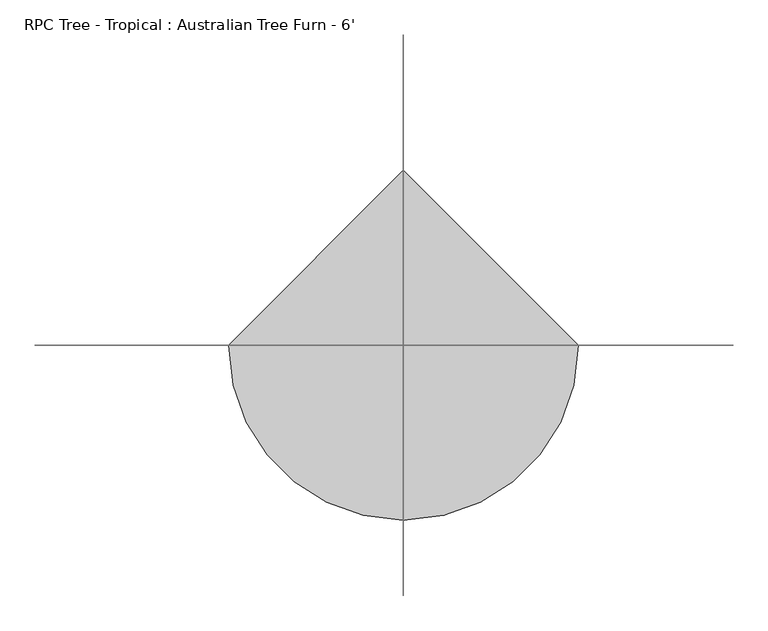
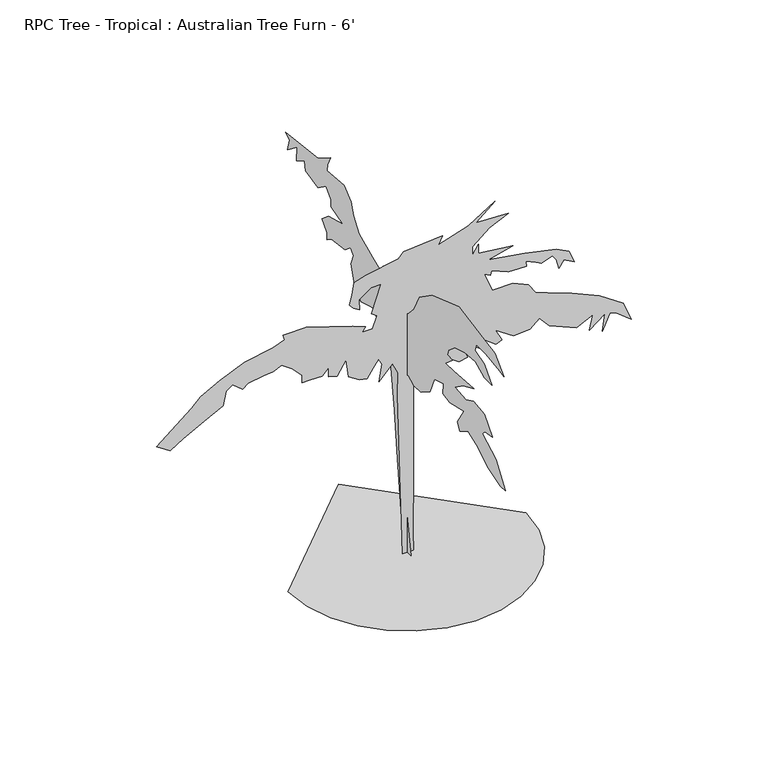
"""IFC4 building model written with IfcOpenShell, lengths in millimetres: geographic element geometry, RPC Tree - Tropical : Australian Tree Furn - 6'."""

from ifc_helpers import new_model, si_unit, origin, place, context, project, spatial, triangles, source, transform, mapped, element, save


def rpc_tree_tropical_australian_tree_furn_6_77f1a640(model_context):
    return source(origin(), model_context, "Body", "Tessellation", [
        triangles([(-639.0365753, 0.0, 0.0007159), (-622.1405136, -146.4247652, 0.0007159), (-574.0277527, -280.8912123, 0.0007159), (-498.5465315, -399.5499215, 0.0007159), (-399.5499215, -498.5465315, 0.0007159), (-280.8912123, -574.0277527, 0.0007159), (-146.4247652, -622.1405136, 0.0007159), (2.79e-05, -639.0365753, 0.0007159), (146.4247652, -622.1429844, 0.0007159), (280.8912123, -574.0277527, 0.0007159), (399.5499215, -498.5465315, 0.0007159), (498.5465315, -399.5499215, 0.0007159), (574.0277527, -280.8912123, 0.0007159), (622.1405136, -146.4247652, 0.0007159), (639.0365753, 5.59e-05, 0.0007159), (-8.38e-05, 639.0365753, 0.0007159), (470.2991641, -3.5e-05, 1828.8014534), (368.5593713, -2.98e-05, 1741.5955845), (542.9711454, -2.94e-05, 1734.3285862), (441.231389, -2.66e-05, 1687.0922253), (350.3907492, -2.2e-05, 1610.7880165), (350.3907492, -1.92e-05, 1563.5516556), (383.0932589, -2.22e-05, 1614.4202076), (383.0932589, -1.92e-05, 1563.5516556), (568.4067295, -1.79e-05, 1541.750806), (437.5966181, -1.59e-05, 1509.0482964), (633.8092781, -1.4e-05, 1476.3456413), (800.9540903, -1.18e-05, 1440.0109406), (869.9913008, -9.7e-06, 1403.673769), (899.0591486, -5.5e-06, 1334.6364132), (840.9235256, -7.5e-06, 1367.3389229), (815.4879416, -5.1e-06, 1327.3695602), (800.9540903, -8.4e-06, 1381.8729195), (779.1532408, -1.01e-05, 1410.9406219), (721.015147, -8.8e-06, 1389.1397724), (691.9473719, -9.7e-06, 1403.673769), (637.4440126, -1.12e-05, 1429.1092804), (641.0762037, -9.4e-06, 1400.0414326), (597.4745047, -9.4e-06, 1400.0414326), (542.9711454, -9.7e-06, 1403.673769), (452.1330491, -1.18e-05, 1440.0109406), (448.4983146, -1.03e-05, 1414.5754292), (415.7958049, -1.14e-05, 1432.7440876), (459.4000111, -5.1e-06, 1327.3695602), (568.4067295, -5.1e-06, 1327.3695602), (651.9778639, -2.9e-06, 1291.0347141), (688.3126373, 3e-07, 1236.5313549), (753.7176567, 1.8e-06, 1211.0958435), (884.5252247, 4.9e-06, 1160.2246754), (1033.5014511, 8.7e-06, 1094.8221268), (1160.6767553, 1.39e-05, 1007.6162579), (1204.2784544, 2.02e-05, 902.2417305), (1120.70732, 1.63e-05, 967.6468225), (1088.0048103, 1.59e-05, 974.9137482), (1048.0353024, 2.11e-05, 887.7078793), (1062.5692263, 1.55e-05, 982.1806738), (978.9980919, 1.94e-05, 916.7781979), (997.1666777, 1.44e-05, 1000.3493322), (909.9608088, 1.7e-05, 956.7450897), (764.6193169, 1.33e-05, 1018.5179907), (710.1159576, 9.6e-06, 1080.2882755), (659.2448622, 1.22e-05, 1036.684033), (572.0389206, 1.26e-05, 1029.4171074), (473.9338986, 8.7e-06, 1094.8221268), (510.2686357, 1.26e-05, 1029.4171074), (477.5660897, 1.35e-05, 1014.8831835), (324.9577085, 6.6e-06, 1131.1569002), (419.4305394, 1.44e-05, 1000.3493322), (284.9882369, 8.7e-06, 1094.8221268), (324.9577085, 1.48e-05, 993.0824066), (277.7212749, 1.52e-05, 985.8154083), (190.5151335, 1.16e-05, 1047.5857658), (88.7756132, 9.6e-06, 1080.2882755), (194.1488688, 1.52e-05, 985.8154083), (30.6385209, 1.11e-05, 1054.8526915), (34.2719928, 1.57e-05, 978.5484827), (34.2719928, 3.32e-05, 684.2282936), (34.2719928, 4.84e-05, 429.8801196), (30.6385209, 6.77e-05, 106.4923825), (34.2719928, 7.35e-05, 0.0013276), (-23.8650472, 7.39e-05, 0.0007003), (-52.9336422, 1.98e-05, 909.5111996), (-49.2999159, 1.22e-05, 1036.684033), (-78.3684632, 8.5e-06, 1098.4543905), (-151.0396997, 1.31e-05, 1022.1501818), (-136.5055487, 7.5e-06, 1116.6229763), (-154.6734259, 5.5e-06, 1149.325486), (-183.7417098, 7.9e-06, 1109.3560507), (-216.4437289, 1.07e-05, 1062.1196171), (-256.4132006, 1.03e-05, 1069.3865427), (-314.5512943, 8.1e-06, 1105.7213161), (-329.0852182, 2e-06, 1207.461109), (-376.3216155, 6.6e-06, 1131.1569002), (-423.5580491, 5.7e-06, 1145.6907515), (-423.5580491, 2.7e-06, 1196.5619196), (-456.2580153, 4.9e-06, 1160.2246754), (-518.0283365, 4.9e-06, 1160.2246754), (-565.2647701, 4.9e-06, 1160.2246754), (-565.2647701, 2.3e-06, 1203.8289179), (-619.7706728, -1e-06, 1258.3322044), (-674.2714886, -3.4e-06, 1298.3017124), (-721.5079222, -2.1e-06, 1276.5008629), (-772.3790903, -1.9e-06, 1272.866201), (-855.9502247, -1e-06, 1258.3322044), (-885.0205433, 3e-07, 1236.5313549), (-939.5239025, -2.3e-06, 1280.133054), (-972.2238688, -8e-07, 1254.6975426), (-990.3925272, 3.8e-06, 1178.3933338), (-1092.13232, 6.8e-06, 1127.5247091), (-1204.773773, 1.05e-05, 1065.7543516), (-1273.8110561, 1.31e-05, 1022.1501818), (-1346.4830738, 1.03e-05, 1069.3865427), (-1157.5373394, 1.2e-06, 1221.9975037), (-1110.3009058, -1.9e-06, 1272.866201), (-1008.561113, -5.1e-06, 1327.3695602), (-874.1188105, -8.6e-06, 1385.5075813), (-721.5079222, -1.03e-05, 1414.5754292), (-659.7375647, -1.16e-05, 1436.3762787), (-667.004563, -1.33e-05, 1465.4439812), (-539.8317295, -1.33e-05, 1465.4439812), (-416.2885437, -1.1e-05, 1425.4770893), (-292.7479377, -8.6e-06, 1385.5075813), (-223.7109271, -7.1e-06, 1360.0720699), (-241.8788043, -5.5e-06, 1334.6364132), (-187.3751907, -5.5e-06, 1334.6364132), (-161.9403697, -9.4e-06, 1400.0414326), (-191.0089079, -1.07e-05, 1421.8422821), (-140.1390206, -1.96e-05, 1570.8185085), (-194.6423889, -1.96e-05, 1570.8185085), (-260.0454098, -1.68e-05, 1523.5821476), (-256.4132006, -1.33e-05, 1465.4439812), (-289.1157284, -1.46e-05, 1487.2474468), (-310.9165598, -1.62e-05, 1512.6804874), (-296.3826722, -1.94e-05, 1567.1838467), (-285.4809939, -2.31e-05, 1628.956675), (-220.0774642, -2.44e-05, 1650.7575245), (-45.666444, -2.63e-05, 1683.4600342), (-20.2313959, -2.81e-05, 1712.5277367), (190.5151335, -2.92e-05, 1730.6963951), (168.7137935, -2.66e-05, 1687.0922253), (328.5898996, -2.96e-05, 1737.9633934), (3.03e-05, -861.8582216, 1549.8330162), (2.4e-05, -733.5424347, 1570.5289913), (2.01e-05, -646.6209961, 1570.5289913), (2.06e-05, -630.0627771, 1529.1370411), (2.54e-05, -721.12437, 1504.3009117), (3.07e-05, -787.3523769, 1425.6574562), (2.76e-05, -716.9866865, 1425.6574562), (2.26e-05, -634.2029314, 1467.0492611), (1.86e-05, -539.0011479, 1458.7689526), (1.52e-05, -443.8018716, 1429.7951397), (1.41e-05, -385.8542459, 1380.1253517), (1.46e-05, -373.4361812, 1347.0113846), (1.68e-05, -423.1059328, 1347.0113846), (1.55e-05, -356.8778895, 1289.0637589), (1.89e-05, -435.5239975, 1293.2039131), (2.69e-05, -621.7848667, 1305.6220505), (2.36e-05, -518.3052092, 1260.089946), (2.19e-05, -443.8018716, 1206.2800037), (2.68e-05, -547.2815291, 1198.0020933), (2.89e-05, -617.6471832, 1231.1161331), (3.37e-05, -716.9866865, 1218.6980684), (3.97e-05, -795.6302147, 1135.9143133), (3.69e-05, -725.2645243, 1123.4987921), (3.66e-05, -700.4309383, 1098.6626627), (4.42e-05, -824.6040276, 1028.2969723), (5.2e-05, -915.6656204, 904.1213396), (4.99e-05, -865.9959051, 899.9836561), (4.34e-05, -745.9604994, 937.2353794), (3.69e-05, -642.4808418, 999.3231594), (3.26e-05, -567.9774679, 1032.4371992), (3.06e-05, -489.3313963, 982.7648678), (2.84e-05, -468.6354575, 1024.1567453), (2.82e-05, -530.7232738, 1123.4987921), (2.33e-05, -398.2697671, 1090.3847523), (2e-05, -332.0443036, 1102.802817), (1.84e-05, -336.1819871, 1160.7504427), (1.55e-05, -253.3997399, 1135.9143133), (1.65e-05, -212.0081348, 1040.715037), (1.44e-05, -129.2246341, 986.9050947), (1.15e-05, -62.9981487, 982.7648678), (8.4e-06, -13.3280768, 1011.7412241), (6.8e-06, 32.2026538, 999.3231594), (4.5e-06, 52.8985925, 1044.8527205), (4.9e-06, 81.8726461, 986.9050947), (7e-06, 86.0118375, 912.3991774), (1.57e-05, 57.0377794, 664.0505281), (2.77e-05, 19.7852431, 316.3597959), (3.93e-05, -34.0238362, 0.0007149), (3.64e-05, 36.3418406, 0.0), (3.07e-05, 52.8985925, 167.3503229), (1.97e-05, 90.1512742, 477.7870791), (1.08e-05, 119.1250779, 734.4162186), (1.5e-06, 156.3777732, 991.0453217), (-4.8e-06, 210.1869524, 1119.3585651), (-7.3e-06, 268.135323, 1119.3585651), (-1.14e-05, 305.3869918, 1198.0020933), (-1.38e-05, 371.6149987, 1181.4464178), (-1.58e-05, 429.5625881, 1160.7504427), (-2.04e-05, 491.6504045, 1222.8382954), (-2.47e-05, 520.6242173, 1322.177726), (-2.55e-05, 499.9282785, 1380.1253517), (-2.76e-05, 528.9020914, 1409.0991646), (-2.86e-05, 578.5718067, 1367.7072144), (-3.37e-05, 702.7474394, 1351.1515388), (-3.47e-05, 744.1393169, 1322.177726), (-3.59e-05, 744.1393169, 1363.5696762), (-3.96e-05, 793.8090322, 1413.2393188), (-3.83e-05, 731.7212523, 1462.9091068), (-3.35e-05, 599.2677455, 1500.1607574), (-3.93e-05, 706.8876663, 1533.2747246), (-4.06e-05, 711.0252771, 1570.5289913), (-4.41e-05, 756.5573816, 1620.1987793), (-4.58e-05, 831.0607555, 1566.3888371), (-5.18e-05, 946.9584778, 1591.2223503), (-5.36e-05, 955.2363155, 1640.8946091), (-5.57e-05, 1029.7422329, 1599.5028042), (-5.79e-05, 1025.602006, 1678.1462597), (-5.98e-05, 1112.525988, 1611.9183254), (-6.09e-05, 1095.9676964, 1674.0061054), (-6.33e-05, 1133.2218904, 1698.8422348), (-5.08e-05, 831.0607555, 1731.9562019), (-4.78e-05, 715.1655041, 1806.4596485), (-4.73e-05, 739.99909, 1752.652177), (-4.64e-05, 748.2795439, 1711.2603722), (-3.97e-05, 586.8496808, 1727.8160477), (-3.52e-05, 520.6242173, 1674.0061054), (-3.23e-05, 499.9282785, 1607.7806419), (-2.78e-05, 446.1183363, 1537.4150242), (-2.05e-05, 321.9452471, 1479.4647823), (-1.04e-05, 143.960199, 1409.0991646), (-1.65e-05, 226.7434454, 1487.7452362), (-9.7e-06, 114.9858956, 1429.7951397), (-2.2e-06, -0.9105653, 1351.1515388), (-1.4e-06, -62.9981487, 1417.3796185), (-2.2e-06, -112.668141, 1516.7190491), (7e-07, -232.7038011, 1599.5028042), (9.2e-06, -481.0535222, 1686.4242428), (2.03e-05, -700.4309383, 1645.0322926), (2.61e-05, -816.3261898, 1624.3363174), (3.23e-05, -899.1099449, 1541.5525623)], [[15, 16, 1], [14, 15, 1], [14, 1, 2], [13, 14, 2], [13, 2, 3], [13, 3, 4], [12, 13, 4], [11, 12, 4], [11, 4, 5], [11, 5, 6], [11, 6, 7], [11, 7, 8], [11, 8, 9], [11, 9, 10], [141, 17, 18], [54, 55, 56], [73, 74, 75], [67, 68, 69], [24, 25, 26], [18, 19, 20], [51, 52, 53], [22, 23, 24], [84, 85, 86], [29, 30, 31], [56, 57, 58], [31, 32, 33], [130, 131, 132], [138, 139, 140], [41, 42, 43], [111, 112, 113], [110, 111, 113], [109, 110, 113], [122, 123, 124], [118, 119, 120], [18, 20, 21], [141, 18, 21], [69, 70, 71], [69, 71, 72], [28, 29, 31], [28, 31, 33], [28, 33, 34], [27, 28, 34], [27, 34, 35], [27, 35, 36], [27, 36, 37], [130, 132, 133], [130, 133, 134], [50, 51, 53], [50, 53, 54], [50, 54, 56], [50, 56, 58], [140, 141, 21], [37, 38, 39], [64, 65, 66], [64, 66, 67], [80, 81, 82], [79, 80, 82], [78, 79, 82], [77, 78, 82], [76, 77, 82], [76, 82, 83], [75, 76, 83], [97, 98, 99], [49, 50, 58], [49, 58, 59], [49, 59, 60], [48, 49, 60], [48, 60, 61], [47, 48, 61], [129, 130, 134], [129, 134, 135], [129, 135, 136], [129, 136, 137], [128, 129, 137], [108, 109, 113], [108, 113, 114], [107, 108, 114], [107, 114, 115], [106, 107, 115], [106, 115, 116], [105, 106, 116], [104, 105, 116], [103, 104, 116], [103, 116, 117], [102, 103, 117], [101, 102, 117], [101, 117, 118], [75, 83, 84], [26, 27, 37], [26, 37, 39], [26, 39, 40], [26, 40, 41], [26, 41, 43], [92, 93, 94], [92, 94, 95], [126, 127, 128], [101, 118, 120], [100, 101, 120], [100, 120, 121], [99, 100, 121], [97, 99, 121], [96, 97, 121], [95, 96, 121], [95, 121, 122], [92, 95, 122], [92, 122, 124], [140, 21, 22], [88, 89, 90], [24, 26, 43], [22, 24, 43], [88, 90, 91], [88, 91, 92], [88, 92, 124], [87, 88, 124], [87, 124, 125], [47, 61, 62], [47, 62, 63], [47, 63, 64], [46, 47, 64], [45, 46, 64], [44, 45, 64], [44, 64, 67], [43, 44, 67], [137, 138, 140], [128, 137, 140], [126, 128, 140], [126, 140, 22], [126, 22, 43], [126, 43, 67], [126, 67, 69], [126, 69, 72], [126, 72, 73], [125, 126, 73], [87, 125, 73], [87, 73, 75], [87, 75, 84], [87, 84, 86], [231, 232, 233], [156, 157, 158], [240, 241, 142], [222, 223, 224], [218, 219, 220], [220, 221, 222], [218, 220, 222], [153, 154, 155], [240, 142, 143], [239, 240, 143], [146, 147, 148], [205, 206, 207], [162, 163, 164], [156, 158, 159], [216, 217, 218], [216, 218, 222], [166, 167, 168], [166, 168, 169], [222, 224, 225], [239, 143, 144], [238, 239, 144], [146, 148, 149], [145, 146, 149], [165, 166, 169], [165, 169, 170], [207, 208, 209], [188, 189, 190], [188, 190, 191], [188, 191, 192], [187, 188, 192], [187, 192, 193], [186, 187, 193], [186, 193, 194], [185, 186, 194], [171, 172, 173], [171, 173, 174], [145, 149, 150], [155, 156, 159], [165, 170, 171], [165, 171, 174], [175, 176, 177], [182, 183, 184], [205, 207, 209], [205, 209, 210], [204, 205, 210], [203, 204, 210], [161, 162, 164], [161, 164, 165], [161, 165, 174], [160, 161, 174], [159, 160, 174], [159, 174, 175], [159, 175, 177], [155, 159, 177], [238, 144, 145], [238, 145, 150], [237, 238, 150], [237, 150, 151], [237, 151, 152], [236, 237, 152], [235, 236, 152], [235, 152, 153], [235, 153, 155], [235, 155, 177], [235, 177, 178], [234, 235, 178], [234, 178, 179], [234, 179, 180], [234, 180, 181], [234, 181, 182], [234, 182, 184], [231, 233, 234], [231, 234, 184], [214, 215, 216], [214, 216, 222], [213, 214, 222], [213, 222, 225], [213, 225, 226], [212, 213, 226], [212, 226, 227], [212, 227, 228], [211, 212, 228], [210, 211, 228], [210, 228, 229], [203, 210, 229], [203, 229, 230], [202, 203, 230], [184, 185, 194], [184, 194, 195], [231, 184, 195], [230, 231, 195], [230, 195, 196], [230, 196, 197], [202, 230, 197], [202, 197, 198], [201, 202, 198], [200, 201, 198], [199, 200, 198]], closed=False),
    ])


if __name__ == "__main__":
    model = new_model("IFC4")
    model_context = context("Model", 3, world=origin())
    ifc_project = project(units=[si_unit("LENGTHUNIT", "METRE", prefix="MILLI")], contexts=[model_context])
    site = spatial("IfcSite", under=ifc_project)
    building = spatial("IfcBuilding", under=site)
    placement = place(None, origin())
    rpc_tree_tropical_australian_tree_furn_6_shape = rpc_tree_tropical_australian_tree_furn_6_77f1a640(model_context)
    element("IfcGeographicElement", 1, ObjectType="RPC Tree - Tropical : Australian Tree Furn - 6'", at=placement, inside=building, context=model_context, shape_type="MappedRepresentation", body=[
        mapped(rpc_tree_tropical_australian_tree_furn_6_shape, transform((0.0, 0.0, 0.0), x_axis=(1.0, 0.0, 0.0), y_axis=(0.0, 1.0, 0.0), z_axis=(0.0, 0.0, 1.0))),
    ])
    save(model, "model.ifc")

# Revit data of these elements
# Type "RPC Tree - Tropical : Australian Tree Furn - 6'"
#   built-in parameter 1005198 = "{2, 15},{39, RPC-16-FVCN-UWG0-AP53-A000-ST1L-LVER-AU},{1, 0},{1, 0},{2, 35},{1, 8},{5, Color},{1, 0},{1, 0},{3, 0.8},{3, 0.8},{3, 0.8},{1, 8},{7, BBoxMin},{1, 0},{1, 0},{1, 0},{1, 0},{1, 0},{1, 8},{7, BBoxMax},{1, 0},{1, 0},{1, 0},{1, 0},{1, 0},{2, 11},{9, RPCTypeId},{1, 0},{1, 0},{39, RPC-16-FVCN-UWG0-AP53-A000-ST1L-LVER-AU},{1, 6},{14, RPCPlantHeight},{1, 0},{1, 0},{1, 6},{2, 11},{7, keyword},{1, 0},{1, 0},{99, :Geometry:RPC:Australian Tree Fern:Alsophila cooperi (Cyathea australis):Sydney:Tree fern:Tropical.},{2, 11},{8, category},{1, 0},{1, 0},{17, :Trees [Tropical]},{2, 11},{12, LocalizedUID},{1, 0},{1, 0},{20, Australian Tree Fern},{2, 14},{6, Height},{1, 0},{1, 0},{1, 6},{1, 2},{16, Cast Reflections},{1, 0},{1, 0},{1, 0},{1, 2},{12, Cast Shadows},{1, 0},{1, 0},{1, 1},{1, 2},{9, Lock View},{1, 0},{1, 0},{1, 0},{1, 4},{5, ViewC},{1, 0},{1, 0},{1, 0},{2, 11},{20, AdvancedUIDefinition},{1, 0},{1, 0},{0, },{2, 11},{10, AssetLibID},{1, 0},{1, 0},{36, 4D3F6E72-3F99-4203-98E9-AF80B3C7A7A4},{2, 11},{10, BaseSchema},{1, 0},{1, 0},{9, RPCSchema},{2, 11},{12, ExchangeGUID},{1, 0},{1, 0},{0, },{1, 2},{6, Hidden},{1, 0},{1, 0},{1, 0},{1, 4},{11, RPCCategory},{1, 0},{1, 0},{1, 0},{2, 11},{8, RPCImage},{1, 0},{1, 0},{0, },{1, 4},{13, SchemaVersion},{1, 0},{1, 0},{1, 4},{2, 11},{12, UIDefinition},{1, 0},{1, 0},{0, },{2, 11},{6, UIName},{1, 0},{1, 0},{39, RPC-16-FVCN-UWG0-AP53-A000-ST1L-LVER-AU},{2, 11},{11, VersionGUID},{1, 0},{1, 0},{9, RPCSchema},{2, 11},{9, assettype},{1, 0},{1, 0},{11, RPCGeometry},{2, 11},{11, description},{1, 0},{1, 0},{0, },{2, 11},{9, localname},{1, 0},{1, 0},{3, RPC},{2, 11},{9, localtype},{1, 0},{1, 0},{3, RPC},{1, 4},{8, revision},{1, 0},{1, 0},{1, 1},{2, 11},{9, thumbnail},{1, 0},{1, 0},{0, },{1, 4},{7, version},{1, 0},{1, 0},{1, 1},{1, 2},{20, RPC_Cast Reflections},{1, 0},{1, 0},{1, 1},{1, 2},{16, RPC_Cast Shadows},{1, 0},{1, 0},{1, 1},{1, 2},{13, RPC_Lock View},{1, 0},{1, 0},{1, 0},{1, 4},{9, RPC_ViewC},{1, 0},{1, 0},{1, 0},{21, assetlibrary_base.fbx},{1, 5},"
#   built-in parameter 1005195 = "RPC-16-FVCN-UWG0-AP53-A000-ST1L-LVER-AU"
#   Type Comments = "Australian Tree Furn"
#   Assembly Code = "G2050500"
#   Height = 1828.8 mm
#   Plan Symbol = element 336060
#   Default Elevation = 0
